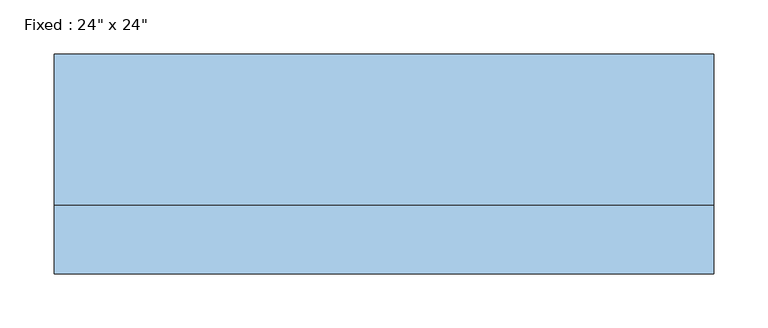
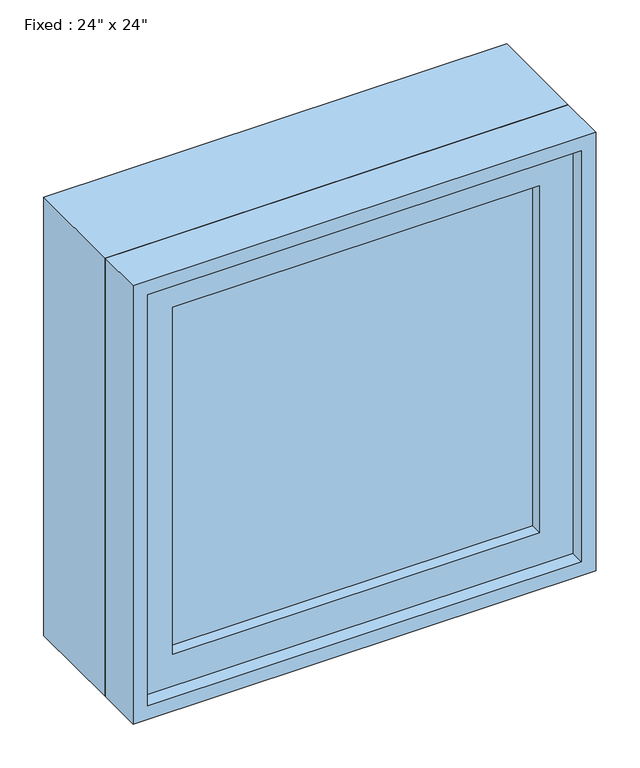
"""IFC4 building model written with IfcOpenShell, lengths in millimetres: window geometry."""

from ifc_helpers import new_model, si_unit, frame, origin, place, context, project, spatial, polyline, outline, extrude, source, transform, mapped, element, save


def window_347e55ac(model_context):
    return source(origin(), model_context, "Body", "SweptSolid", [
        extrude(outline(polyline([(203.2, -53.975), (203.2, -66.675), (-279.4, -66.675), (-279.4, -53.975), (203.2, -53.975)])), frame((0.0, 0.0, 977.9), z_axis=(0.0, 0.0, 1.0), x_axis=(1.0, 0.0, 0.0)), (0.0, 0.0, 1.0), 482.6),
        extrude(outline(polyline([(1504.95, -323.85), (933.45, -323.85), (933.45, 247.65), (1504.95, 247.65), (1504.95, -323.85)]), holes=[polyline([(1460.5, -279.4), (1460.5, 203.2), (977.9, 203.2), (977.9, -279.4), (1460.5, -279.4)])]), frame((0.0, -82.55, 0.0), z_axis=(0.0, 1.0, 0.0), x_axis=(0.0, 0.0, 1.0)), (0.0, 0.0, 1.0), 44.45),
        extrude(outline(polyline([(1524.0, -342.9), (914.4, -342.9), (914.4, 266.7), (1524.0, 266.7), (1524.0, -342.9)]), holes=[polyline([(1492.25, -311.15), (1492.25, 234.95), (946.15, 234.95), (946.15, -311.15), (1492.25, -311.15)])]), frame((0.0, -38.1, 0.0), z_axis=(0.0, 1.0, 0.0), x_axis=(0.0, 0.0, 1.0)), (0.0, 0.0, 1.0), 139.7),
        extrude(outline(polyline([(1524.0, 266.7), (1524.0, -342.9), (914.4, -342.9), (914.4, 266.7), (1524.0, 266.7)]), holes=[polyline([(1504.95, 247.65), (933.45, 247.65), (933.45, -323.85), (1504.95, -323.85), (1504.95, 247.65)])]), frame((0.0, -101.6, 0.0), z_axis=(0.0, 1.0, 0.0), x_axis=(0.0, 0.0, 1.0)), (0.0, 0.0, 1.0), 63.5),
    ])


if __name__ == "__main__":
    model = new_model("IFC4")
    model_context = context("Model", 3, world=origin())
    ifc_project = project(units=[si_unit("LENGTHUNIT", "METRE", prefix="MILLI")], contexts=[model_context])
    site = spatial("IfcSite", under=ifc_project)
    building = spatial("IfcBuilding", under=site)
    placement = place(None, origin())
    window_shape = window_347e55ac(model_context)
    element("IfcWindow", 1, ObjectType="Fixed : 24\" x 24\"", at=placement, inside=building, context=model_context, shape_type="MappedRepresentation", body=[
        mapped(window_shape, transform((0.0, 0.0, 0.0), x_axis=(1.0, 0.0, 0.0), y_axis=(0.0, 1.0, 0.0), z_axis=(0.0, 0.0, 1.0))),
    ])
    save(model, "model.ifc")

# Revit data of these elements
# Type "Fixed : 24\" x 24\""
#   Type Mark = "3"
#   Construction Type Id = "GSP4R"
#   Assembly Code = "B2020100"
#   Analytic Construction = "1/8 in Pilkington single glazing"
#   Visual Light Transmittance = 0.9
#   Solar Heat Gain Coefficient = 0.78
#   Heat Transfer Coefficient (U) = 0.6496 BTU/(h·ft²·°F)
#   Height = 2' - 0"
#   Default Sill Height = 3' - 0"
#   Width = 2' - 0"
#   Window Inset = 0' - 0 3/4"
#   Define Thermal Properties by = 1
#   Define Thermal Properties by = 1
#   Glass Pane Material = Glass
#   Sash Material = Sash
#   Wall Closure = (empty or 0)
# Element 1 (IfcWindow, "Fixed : 24\" x 24\"")
#   Materials on its faces: "Sash", "Glass"
# Materials
#   "Glass": class "Glass", colour RGB 0 128 192, transparency 0.75, Description = "Soda Lime Glass", Cost = 0
#   "Sash": class "Wood", colour RGB 224 178 126, transparency 0, Cost = 0
